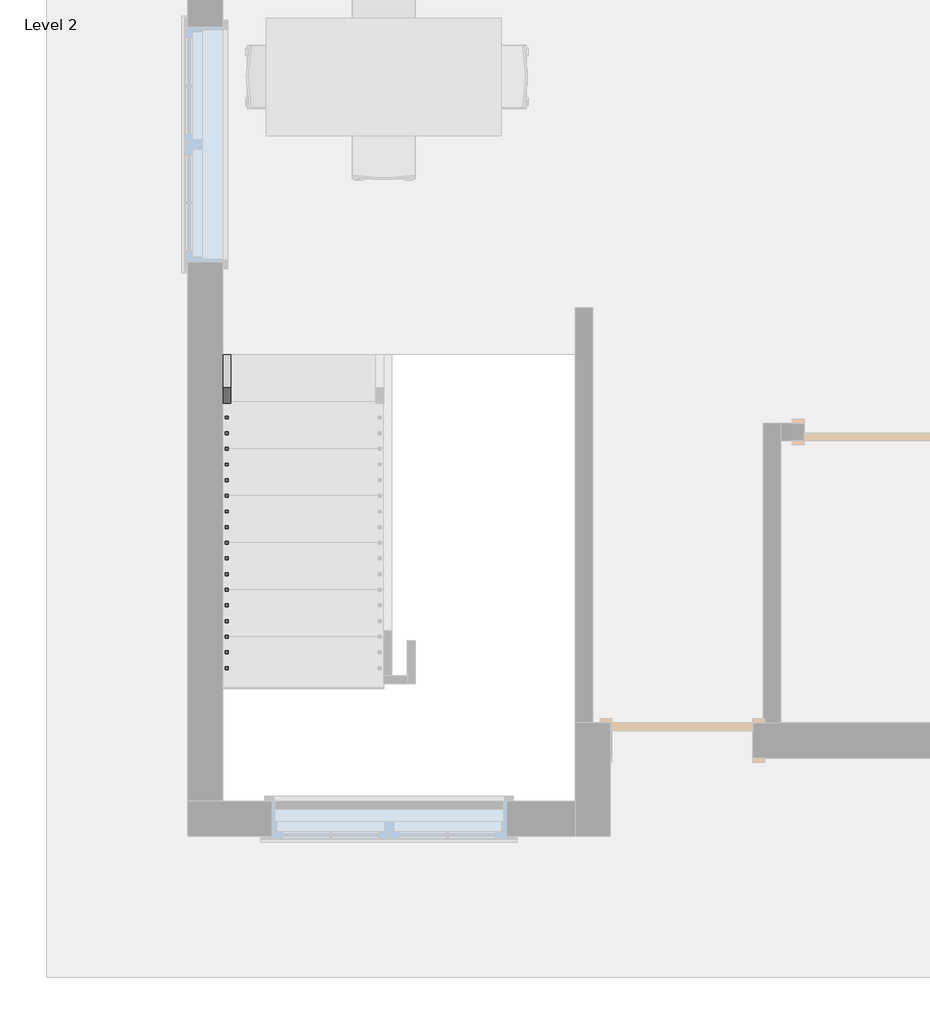
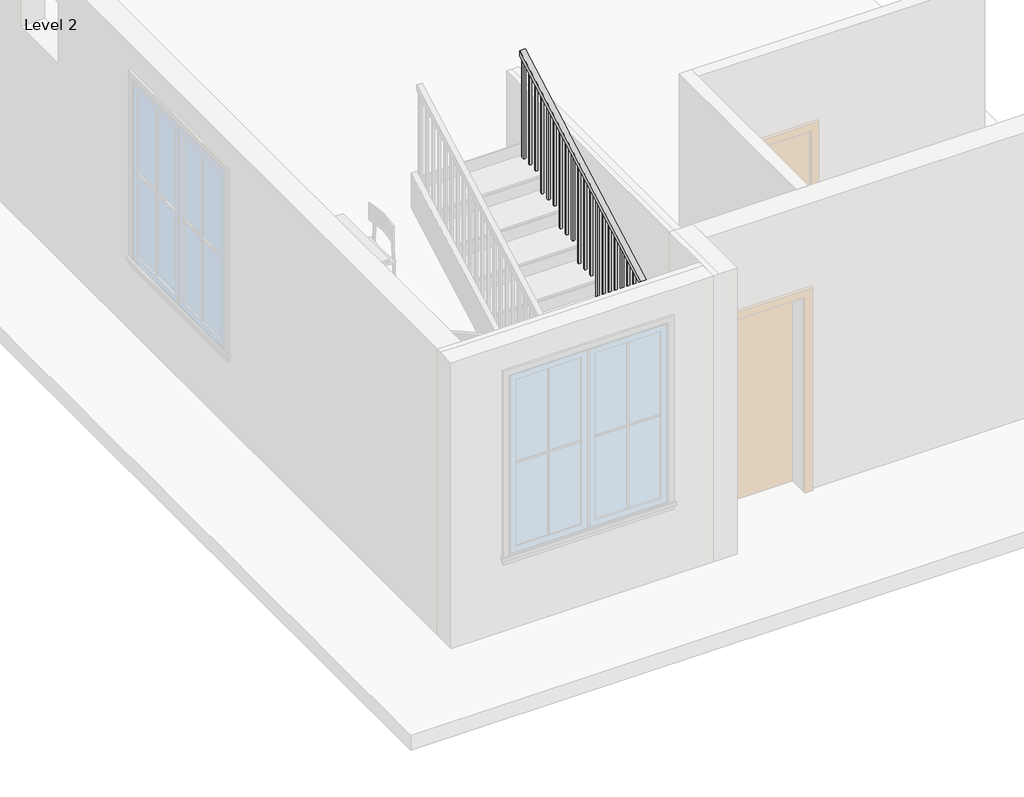
# One storey, part 2 of 3: 1 railing.
"""IFC4 building model written with IfcOpenShell, lengths in millimetres."""

from ifc_helpers import new_model, si_unit, frame, origin, place, context, project, spatial, polyline, outline, extrude, faceted_brep, element, save

model = new_model("IFC4")

# Units and contexts
model_context = context("Model", 3, world=origin())
ifc_project = project(units=[si_unit("LENGTHUNIT", "METRE", prefix="MILLI")], contexts=[model_context])

# Site, building, storey
site = spatial("IfcSite", under=ifc_project)
building = spatial("IfcBuilding", under=site)
storey = spatial("IfcBuildingStorey", under=building, Name="Level 2", Elevation=3048.0)

# Railing
placement = place(None, origin())
element("IfcRailing", 1, ObjectType="Handrail - Rectangular", at=placement, inside=storey, context=model_context, shape_type="SolidModel", body=[
    faceted_brep([(-4181.480864, -3571.6080018, 4131.7333333), (-4181.480864, -3571.6080018, 4073.620221), (-4232.280864, -3571.6080018, 4073.620221), (-4232.280864, -3571.6080018, 4131.7333333), (-4181.480864, -5705.2080018, 5317.0666667), (-4181.480864, -5718.371604, 5266.2666667), (-4232.280864, -5718.371604, 5266.2666667), (-4232.280864, -5705.2080018, 5317.0666667), (-4181.480864, -6416.4080018, 5317.0666667), (-4181.480864, -6416.4080018, 5266.2666667), (-4232.280864, -6467.2080018, 5266.2666667), (-4232.280864, -6467.2080018, 5317.0666667), (-1997.080864, -6416.4080018, 5317.0666667), (-1997.080864, -6416.4080018, 5266.2666667), (-1946.280864, -6467.2080018, 5266.2666667), (-1946.280864, -6467.2080018, 5317.0666667), (-1997.080864, -5705.2080018, 5317.0666667), (-1997.080864, -5692.0443995, 5266.2666667), (-1946.280864, -5692.0443995, 5266.2666667), (-1946.280864, -5705.2080018, 5317.0666667), (-1997.080864, -3571.6080018, 6502.4), (-1946.280864, -3571.6080018, 6502.4), (-1946.280864, -3571.6080018, 6444.2868876), (-1997.080864, -3571.6080018, 6444.2868876)], [[[0, 1, 2, 3]], [[1, 0, 4, 5]], [[2, 1, 5, 6]], [[3, 2, 6, 7]], [[0, 3, 7, 4]], [[5, 4, 8, 9]], [[6, 5, 9, 10]], [[7, 6, 10, 11]], [[4, 7, 11, 8]], [[9, 8, 12, 13]], [[10, 9, 13, 14]], [[11, 10, 14, 15]], [[8, 11, 15, 12]], [[13, 12, 16, 17]], [[14, 13, 17, 18]], [[15, 14, 18, 19]], [[12, 15, 19, 16]], [[20, 21, 22, 23]], [[17, 16, 20, 23]], [[18, 17, 23, 22]], [[19, 18, 22, 21]], [[16, 19, 21, 20]]]),
    extrude(outline(polyline([(-3606.5330018, 6424.8841099), (-3587.4830018, 6435.4674432), (-3587.4830018, 5418.6666667), (-3606.5330018, 5418.6666667), (-3606.5330018, 6424.8841099)])), frame((-1981.205864, 0.0, 0.0), z_axis=(1.0, 0.0, 0.0), x_axis=(0.0, 1.0, 0.0)), (0.0, 0.0, 1.0), 19.05),
    extrude(outline(polyline([(-3708.1330018, 6368.4396654), (-3689.0830018, 6379.0229988), (-3689.0830018, 5418.6666667), (-3708.1330018, 5418.6666667), (-3708.1330018, 6368.4396654)])), frame((-1981.205864, 0.0, 0.0), z_axis=(1.0, 0.0, 0.0), x_axis=(0.0, 1.0, 0.0)), (0.0, 0.0, 1.0), 19.05),
    extrude(outline(polyline([(-3809.7330018, 6311.995221), (-3790.6830018, 6322.5785543), (-3790.6830018, 5418.6666667), (-3809.7330018, 5418.6666667), (-3809.7330018, 6311.995221)])), frame((-1981.205864, 0.0, 0.0), z_axis=(1.0, 0.0, 0.0), x_axis=(0.0, 1.0, 0.0)), (0.0, 0.0, 1.0), 19.05),
    extrude(outline(polyline([(-3911.3330018, 6255.5507765), (-3892.2830018, 6266.1341099), (-3892.2830018, 5249.3333333), (-3911.3330018, 5249.3333333), (-3911.3330018, 6255.5507765)])), frame((-1981.205864, 0.0, 0.0), z_axis=(1.0, 0.0, 0.0), x_axis=(0.0, 1.0, 0.0)), (0.0, 0.0, 1.0), 19.05),
    extrude(outline(polyline([(-4012.9330018, 6199.1063321), (-3993.8830018, 6209.6896654), (-3993.8830018, 5249.3333333), (-4012.9330018, 5249.3333333), (-4012.9330018, 6199.1063321)])), frame((-1981.205864, 0.0, 0.0), z_axis=(1.0, 0.0, 0.0), x_axis=(0.0, 1.0, 0.0)), (0.0, 0.0, 1.0), 19.05),
    extrude(outline(polyline([(-4114.5330018, 6142.6618876), (-4095.4830018, 6153.245221), (-4095.4830018, 5249.3333333), (-4114.5330018, 5249.3333333), (-4114.5330018, 6142.6618876)])), frame((-1981.205864, 0.0, 0.0), z_axis=(1.0, 0.0, 0.0), x_axis=(0.0, 1.0, 0.0)), (0.0, 0.0, 1.0), 19.05),
    extrude(outline(polyline([(-4216.1330018, 6086.2174432), (-4197.0830018, 6096.8007765), (-4197.0830018, 5080.0), (-4216.1330018, 5080.0), (-4216.1330018, 6086.2174432)])), frame((-1981.205864, 0.0, 0.0), z_axis=(1.0, 0.0, 0.0), x_axis=(0.0, 1.0, 0.0)), (0.0, 0.0, 1.0), 19.05),
    extrude(outline(polyline([(-4317.7330018, 6029.7729988), (-4298.6830018, 6040.3563321), (-4298.6830018, 5080.0), (-4317.7330018, 5080.0), (-4317.7330018, 6029.7729988)])), frame((-1981.205864, 0.0, 0.0), z_axis=(1.0, 0.0, 0.0), x_axis=(0.0, 1.0, 0.0)), (0.0, 0.0, 1.0), 19.05),
    extrude(outline(polyline([(-4419.3330018, 5973.3285543), (-4400.2830018, 5983.9118876), (-4400.2830018, 5080.0), (-4419.3330018, 5080.0), (-4419.3330018, 5973.3285543)])), frame((-1981.205864, 0.0, 0.0), z_axis=(1.0, 0.0, 0.0), x_axis=(0.0, 1.0, 0.0)), (0.0, 0.0, 1.0), 19.05),
    extrude(outline(polyline([(-4520.9330018, 5916.8841099), (-4501.8830018, 5927.4674432), (-4501.8830018, 4910.6666667), (-4520.9330018, 4910.6666667), (-4520.9330018, 5916.8841099)])), frame((-1981.205864, 0.0, 0.0), z_axis=(1.0, 0.0, 0.0), x_axis=(0.0, 1.0, 0.0)), (0.0, 0.0, 1.0), 19.05),
    extrude(outline(polyline([(-4622.5330018, 5860.4396654), (-4603.4830018, 5871.0229988), (-4603.4830018, 4910.6666667), (-4622.5330018, 4910.6666667), (-4622.5330018, 5860.4396654)])), frame((-1981.205864, 0.0, 0.0), z_axis=(1.0, 0.0, 0.0), x_axis=(0.0, 1.0, 0.0)), (0.0, 0.0, 1.0), 19.05),
    extrude(outline(polyline([(-4724.1330018, 5803.995221), (-4705.0830018, 5814.5785543), (-4705.0830018, 4910.6666667), (-4724.1330018, 4910.6666667), (-4724.1330018, 5803.995221)])), frame((-1981.205864, 0.0, 0.0), z_axis=(1.0, 0.0, 0.0), x_axis=(0.0, 1.0, 0.0)), (0.0, 0.0, 1.0), 19.05),
    extrude(outline(polyline([(-4825.7330018, 5747.5507765), (-4806.6830018, 5758.1341099), (-4806.6830018, 4741.3333333), (-4825.7330018, 4741.3333333), (-4825.7330018, 5747.5507765)])), frame((-1981.205864, 0.0, 0.0), z_axis=(1.0, 0.0, 0.0), x_axis=(0.0, 1.0, 0.0)), (0.0, 0.0, 1.0), 19.05),
    extrude(outline(polyline([(-4927.3330018, 5691.1063321), (-4908.2830018, 5701.6896654), (-4908.2830018, 4741.3333333), (-4927.3330018, 4741.3333333), (-4927.3330018, 5691.1063321)])), frame((-1981.205864, 0.0, 0.0), z_axis=(1.0, 0.0, 0.0), x_axis=(0.0, 1.0, 0.0)), (0.0, 0.0, 1.0), 19.05),
    extrude(outline(polyline([(-5028.9330018, 5634.6618876), (-5009.8830018, 5645.245221), (-5009.8830018, 4741.3333333), (-5028.9330018, 4741.3333333), (-5028.9330018, 5634.6618876)])), frame((-1981.205864, 0.0, 0.0), z_axis=(1.0, 0.0, 0.0), x_axis=(0.0, 1.0, 0.0)), (0.0, 0.0, 1.0), 19.05),
    extrude(outline(polyline([(-5130.5330018, 5578.2174432), (-5111.4830018, 5588.8007765), (-5111.4830018, 4572.0), (-5130.5330018, 4572.0), (-5130.5330018, 5578.2174432)])), frame((-1981.205864, 0.0, 0.0), z_axis=(1.0, 0.0, 0.0), x_axis=(0.0, 1.0, 0.0)), (0.0, 0.0, 1.0), 19.05),
    extrude(outline(polyline([(-5232.1330018, 5521.7729988), (-5213.0830018, 5532.3563321), (-5213.0830018, 4572.0), (-5232.1330018, 4572.0), (-5232.1330018, 5521.7729988)])), frame((-1981.205864, 0.0, 0.0), z_axis=(1.0, 0.0, 0.0), x_axis=(0.0, 1.0, 0.0)), (0.0, 0.0, 1.0), 19.05),
    extrude(outline(polyline([(-5333.7330018, 5465.3285543), (-5314.6830018, 5475.9118876), (-5314.6830018, 4572.0), (-5333.7330018, 4572.0), (-5333.7330018, 5465.3285543)])), frame((-1981.205864, 0.0, 0.0), z_axis=(1.0, 0.0, 0.0), x_axis=(0.0, 1.0, 0.0)), (0.0, 0.0, 1.0), 19.05),
    extrude(outline(polyline([(-5435.3330018, 5408.8841099), (-5416.2830018, 5419.4674432), (-5416.2830018, 4402.6666667), (-5435.3330018, 4402.6666667), (-5435.3330018, 5408.8841099)])), frame((-1981.205864, 0.0, 0.0), z_axis=(1.0, 0.0, 0.0), x_axis=(0.0, 1.0, 0.0)), (0.0, 0.0, 1.0), 19.05),
    extrude(outline(polyline([(-5536.9330018, 5352.4396654), (-5517.8830018, 5363.0229988), (-5517.8830018, 4402.6666667), (-5536.9330018, 4402.6666667), (-5536.9330018, 5352.4396654)])), frame((-1981.205864, 0.0, 0.0), z_axis=(1.0, 0.0, 0.0), x_axis=(0.0, 1.0, 0.0)), (0.0, 0.0, 1.0), 19.05),
    extrude(outline(polyline([(-5638.5330018, 5295.995221), (-5619.4830018, 5306.5785543), (-5619.4830018, 4402.6666667), (-5638.5330018, 4402.6666667), (-5638.5330018, 5295.995221)])), frame((-1981.205864, 0.0, 0.0), z_axis=(1.0, 0.0, 0.0), x_axis=(0.0, 1.0, 0.0)), (0.0, 0.0, 1.0), 19.05),
    extrude(outline(polyline([(-1962.155864, -5740.1330018), (-1981.205864, -5740.1330018), (-1981.205864, -5721.0830018), (-1962.155864, -5721.0830018), (-1962.155864, -5740.1330018)])), frame((0.0, 0.0, 4402.6666667), z_axis=(0.0, 0.0, 1.0), x_axis=(1.0, 0.0, 0.0)), (0.0, 0.0, 1.0), 863.6),
    extrude(outline(polyline([(-1962.155864, -5841.7330018), (-1981.205864, -5841.7330018), (-1981.205864, -5822.6830018), (-1962.155864, -5822.6830018), (-1962.155864, -5841.7330018)])), frame((0.0, 0.0, 4402.6666667), z_axis=(0.0, 0.0, 1.0), x_axis=(1.0, 0.0, 0.0)), (0.0, 0.0, 1.0), 863.6),
    extrude(outline(polyline([(-1962.155864, -5943.3330018), (-1981.205864, -5943.3330018), (-1981.205864, -5924.2830018), (-1962.155864, -5924.2830018), (-1962.155864, -5943.3330018)])), frame((0.0, 0.0, 4402.6666667), z_axis=(0.0, 0.0, 1.0), x_axis=(1.0, 0.0, 0.0)), (0.0, 0.0, 1.0), 863.6),
    extrude(outline(polyline([(-1962.155864, -6044.9330018), (-1981.205864, -6044.9330018), (-1981.205864, -6025.8830018), (-1962.155864, -6025.8830018), (-1962.155864, -6044.9330018)])), frame((0.0, 0.0, 4402.6666667), z_axis=(0.0, 0.0, 1.0), x_axis=(1.0, 0.0, 0.0)), (0.0, 0.0, 1.0), 863.6),
    extrude(outline(polyline([(-1962.155864, -6146.5330018), (-1981.205864, -6146.5330018), (-1981.205864, -6127.4830018), (-1962.155864, -6127.4830018), (-1962.155864, -6146.5330018)])), frame((0.0, 0.0, 4402.6666667), z_axis=(0.0, 0.0, 1.0), x_axis=(1.0, 0.0, 0.0)), (0.0, 0.0, 1.0), 863.6),
    extrude(outline(polyline([(-1962.155864, -6248.1330018), (-1981.205864, -6248.1330018), (-1981.205864, -6229.0830018), (-1962.155864, -6229.0830018), (-1962.155864, -6248.1330018)])), frame((0.0, 0.0, 4402.6666667), z_axis=(0.0, 0.0, 1.0), x_axis=(1.0, 0.0, 0.0)), (0.0, 0.0, 1.0), 863.6),
    extrude(outline(polyline([(-1962.155864, -6349.7330018), (-1981.205864, -6349.7330018), (-1981.205864, -6330.6830018), (-1962.155864, -6330.6830018), (-1962.155864, -6349.7330018)])), frame((0.0, 0.0, 4402.6666667), z_axis=(0.0, 0.0, 1.0), x_axis=(1.0, 0.0, 0.0)), (0.0, 0.0, 1.0), 863.6),
    extrude(outline(polyline([(-2082.805864, -6451.3330018), (-2082.805864, -6432.2830018), (-2063.755864, -6432.2830018), (-2063.755864, -6451.3330018), (-2082.805864, -6451.3330018)])), frame((0.0, 0.0, 4402.6666667), z_axis=(0.0, 0.0, 1.0), x_axis=(1.0, 0.0, 0.0)), (0.0, 0.0, 1.0), 863.6),
    extrude(outline(polyline([(-2184.405864, -6451.3330018), (-2184.405864, -6432.2830018), (-2165.355864, -6432.2830018), (-2165.355864, -6451.3330018), (-2184.405864, -6451.3330018)])), frame((0.0, 0.0, 4402.6666667), z_axis=(0.0, 0.0, 1.0), x_axis=(1.0, 0.0, 0.0)), (0.0, 0.0, 1.0), 863.6),
    extrude(outline(polyline([(-2286.005864, -6451.3330018), (-2286.005864, -6432.2830018), (-2266.955864, -6432.2830018), (-2266.955864, -6451.3330018), (-2286.005864, -6451.3330018)])), frame((0.0, 0.0, 4402.6666667), z_axis=(0.0, 0.0, 1.0), x_axis=(1.0, 0.0, 0.0)), (0.0, 0.0, 1.0), 863.6),
    extrude(outline(polyline([(-2387.605864, -6451.3330018), (-2387.605864, -6432.2830018), (-2368.555864, -6432.2830018), (-2368.555864, -6451.3330018), (-2387.605864, -6451.3330018)])), frame((0.0, 0.0, 4402.6666667), z_axis=(0.0, 0.0, 1.0), x_axis=(1.0, 0.0, 0.0)), (0.0, 0.0, 1.0), 863.6),
    extrude(outline(polyline([(-2489.205864, -6451.3330018), (-2489.205864, -6432.2830018), (-2470.155864, -6432.2830018), (-2470.155864, -6451.3330018), (-2489.205864, -6451.3330018)])), frame((0.0, 0.0, 4402.6666667), z_axis=(0.0, 0.0, 1.0), x_axis=(1.0, 0.0, 0.0)), (0.0, 0.0, 1.0), 863.6),
    extrude(outline(polyline([(-2590.805864, -6451.3330018), (-2590.805864, -6432.2830018), (-2571.755864, -6432.2830018), (-2571.755864, -6451.3330018), (-2590.805864, -6451.3330018)])), frame((0.0, 0.0, 4402.6666667), z_axis=(0.0, 0.0, 1.0), x_axis=(1.0, 0.0, 0.0)), (0.0, 0.0, 1.0), 863.6),
    extrude(outline(polyline([(-2692.405864, -6451.3330018), (-2692.405864, -6432.2830018), (-2673.355864, -6432.2830018), (-2673.355864, -6451.3330018), (-2692.405864, -6451.3330018)])), frame((0.0, 0.0, 4402.6666667), z_axis=(0.0, 0.0, 1.0), x_axis=(1.0, 0.0, 0.0)), (0.0, 0.0, 1.0), 863.6),
    extrude(outline(polyline([(-2794.005864, -6451.3330018), (-2794.005864, -6432.2830018), (-2774.955864, -6432.2830018), (-2774.955864, -6451.3330018), (-2794.005864, -6451.3330018)])), frame((0.0, 0.0, 4402.6666667), z_axis=(0.0, 0.0, 1.0), x_axis=(1.0, 0.0, 0.0)), (0.0, 0.0, 1.0), 863.6),
    extrude(outline(polyline([(-2895.605864, -6451.3330018), (-2895.605864, -6432.2830018), (-2876.555864, -6432.2830018), (-2876.555864, -6451.3330018), (-2895.605864, -6451.3330018)])), frame((0.0, 0.0, 4402.6666667), z_axis=(0.0, 0.0, 1.0), x_axis=(1.0, 0.0, 0.0)), (0.0, 0.0, 1.0), 863.6),
    extrude(outline(polyline([(-2997.205864, -6451.3330018), (-2997.205864, -6432.2830018), (-2978.155864, -6432.2830018), (-2978.155864, -6451.3330018), (-2997.205864, -6451.3330018)])), frame((0.0, 0.0, 4402.6666667), z_axis=(0.0, 0.0, 1.0), x_axis=(1.0, 0.0, 0.0)), (0.0, 0.0, 1.0), 863.6),
    extrude(outline(polyline([(-3098.805864, -6451.3330018), (-3098.805864, -6432.2830018), (-3079.755864, -6432.2830018), (-3079.755864, -6451.3330018), (-3098.805864, -6451.3330018)])), frame((0.0, 0.0, 4402.6666667), z_axis=(0.0, 0.0, 1.0), x_axis=(1.0, 0.0, 0.0)), (0.0, 0.0, 1.0), 863.6),
    extrude(outline(polyline([(-3200.405864, -6451.3330018), (-3200.405864, -6432.2830018), (-3181.355864, -6432.2830018), (-3181.355864, -6451.3330018), (-3200.405864, -6451.3330018)])), frame((0.0, 0.0, 4402.6666667), z_axis=(0.0, 0.0, 1.0), x_axis=(1.0, 0.0, 0.0)), (0.0, 0.0, 1.0), 863.6),
    extrude(outline(polyline([(-3302.005864, -6451.3330018), (-3302.005864, -6432.2830018), (-3282.955864, -6432.2830018), (-3282.955864, -6451.3330018), (-3302.005864, -6451.3330018)])), frame((0.0, 0.0, 4402.6666667), z_axis=(0.0, 0.0, 1.0), x_axis=(1.0, 0.0, 0.0)), (0.0, 0.0, 1.0), 863.6),
    extrude(outline(polyline([(-3403.605864, -6451.3330018), (-3403.605864, -6432.2830018), (-3384.555864, -6432.2830018), (-3384.555864, -6451.3330018), (-3403.605864, -6451.3330018)])), frame((0.0, 0.0, 4402.6666667), z_axis=(0.0, 0.0, 1.0), x_axis=(1.0, 0.0, 0.0)), (0.0, 0.0, 1.0), 863.6),
    extrude(outline(polyline([(-3505.205864, -6451.3330018), (-3505.205864, -6432.2830018), (-3486.155864, -6432.2830018), (-3486.155864, -6451.3330018), (-3505.205864, -6451.3330018)])), frame((0.0, 0.0, 4402.6666667), z_axis=(0.0, 0.0, 1.0), x_axis=(1.0, 0.0, 0.0)), (0.0, 0.0, 1.0), 863.6),
    extrude(outline(polyline([(-3606.805864, -6451.3330018), (-3606.805864, -6432.2830018), (-3587.755864, -6432.2830018), (-3587.755864, -6451.3330018), (-3606.805864, -6451.3330018)])), frame((0.0, 0.0, 4402.6666667), z_axis=(0.0, 0.0, 1.0), x_axis=(1.0, 0.0, 0.0)), (0.0, 0.0, 1.0), 863.6),
    extrude(outline(polyline([(-3708.405864, -6451.3330018), (-3708.405864, -6432.2830018), (-3689.355864, -6432.2830018), (-3689.355864, -6451.3330018), (-3708.405864, -6451.3330018)])), frame((0.0, 0.0, 4402.6666667), z_axis=(0.0, 0.0, 1.0), x_axis=(1.0, 0.0, 0.0)), (0.0, 0.0, 1.0), 863.6),
    extrude(outline(polyline([(-3810.005864, -6451.3330018), (-3810.005864, -6432.2830018), (-3790.955864, -6432.2830018), (-3790.955864, -6451.3330018), (-3810.005864, -6451.3330018)])), frame((0.0, 0.0, 4402.6666667), z_axis=(0.0, 0.0, 1.0), x_axis=(1.0, 0.0, 0.0)), (0.0, 0.0, 1.0), 863.6),
    extrude(outline(polyline([(-3911.605864, -6451.3330018), (-3911.605864, -6432.2830018), (-3892.555864, -6432.2830018), (-3892.555864, -6451.3330018), (-3911.605864, -6451.3330018)])), frame((0.0, 0.0, 4402.6666667), z_axis=(0.0, 0.0, 1.0), x_axis=(1.0, 0.0, 0.0)), (0.0, 0.0, 1.0), 863.6),
    extrude(outline(polyline([(-4013.205864, -6451.3330018), (-4013.205864, -6432.2830018), (-3994.155864, -6432.2830018), (-3994.155864, -6451.3330018), (-4013.205864, -6451.3330018)])), frame((0.0, 0.0, 4402.6666667), z_axis=(0.0, 0.0, 1.0), x_axis=(1.0, 0.0, 0.0)), (0.0, 0.0, 1.0), 863.6),
    extrude(outline(polyline([(-4114.805864, -6451.3330018), (-4114.805864, -6432.2830018), (-4095.755864, -6432.2830018), (-4095.755864, -6451.3330018), (-4114.805864, -6451.3330018)])), frame((0.0, 0.0, 4402.6666667), z_axis=(0.0, 0.0, 1.0), x_axis=(1.0, 0.0, 0.0)), (0.0, 0.0, 1.0), 863.6),
    extrude(outline(polyline([(-4216.405864, -6406.8830018), (-4197.355864, -6406.8830018), (-4197.355864, -6425.9330018), (-4216.405864, -6425.9330018), (-4216.405864, -6406.8830018)])), frame((0.0, 0.0, 4402.6666667), z_axis=(0.0, 0.0, 1.0), x_axis=(1.0, 0.0, 0.0)), (0.0, 0.0, 1.0), 863.6),
    extrude(outline(polyline([(-4216.405864, -6305.2830018), (-4197.355864, -6305.2830018), (-4197.355864, -6324.3330018), (-4216.405864, -6324.3330018), (-4216.405864, -6305.2830018)])), frame((0.0, 0.0, 4402.6666667), z_axis=(0.0, 0.0, 1.0), x_axis=(1.0, 0.0, 0.0)), (0.0, 0.0, 1.0), 863.6),
    extrude(outline(polyline([(-4216.405864, -6203.6830018), (-4197.355864, -6203.6830018), (-4197.355864, -6222.7330018), (-4216.405864, -6222.7330018), (-4216.405864, -6203.6830018)])), frame((0.0, 0.0, 4402.6666667), z_axis=(0.0, 0.0, 1.0), x_axis=(1.0, 0.0, 0.0)), (0.0, 0.0, 1.0), 863.6),
    extrude(outline(polyline([(-4216.405864, -6102.0830018), (-4197.355864, -6102.0830018), (-4197.355864, -6121.1330018), (-4216.405864, -6121.1330018), (-4216.405864, -6102.0830018)])), frame((0.0, 0.0, 4402.6666667), z_axis=(0.0, 0.0, 1.0), x_axis=(1.0, 0.0, 0.0)), (0.0, 0.0, 1.0), 863.6),
    extrude(outline(polyline([(-4216.405864, -6000.4830018), (-4197.355864, -6000.4830018), (-4197.355864, -6019.5330018), (-4216.405864, -6019.5330018), (-4216.405864, -6000.4830018)])), frame((0.0, 0.0, 4402.6666667), z_axis=(0.0, 0.0, 1.0), x_axis=(1.0, 0.0, 0.0)), (0.0, 0.0, 1.0), 863.6),
    extrude(outline(polyline([(-4216.405864, -5898.8830018), (-4197.355864, -5898.8830018), (-4197.355864, -5917.9330018), (-4216.405864, -5917.9330018), (-4216.405864, -5898.8830018)])), frame((0.0, 0.0, 4402.6666667), z_axis=(0.0, 0.0, 1.0), x_axis=(1.0, 0.0, 0.0)), (0.0, 0.0, 1.0), 863.6),
    extrude(outline(polyline([(-4216.405864, -5797.2830018), (-4197.355864, -5797.2830018), (-4197.355864, -5816.3330018), (-4216.405864, -5816.3330018), (-4216.405864, -5797.2830018)])), frame((0.0, 0.0, 4402.6666667), z_axis=(0.0, 0.0, 1.0), x_axis=(1.0, 0.0, 0.0)), (0.0, 0.0, 1.0), 863.6),
    extrude(outline(polyline([(-5714.7330018, 5264.245221), (-5695.6830018, 5253.6618876), (-5695.6830018, 4402.6666667), (-5714.7330018, 4402.6666667), (-5714.7330018, 5264.245221)])), frame((-4216.405864, 0.0, 0.0), z_axis=(1.0, 0.0, 0.0), x_axis=(0.0, 1.0, 0.0)), (0.0, 0.0, 1.0), 19.05),
    extrude(outline(polyline([(-5613.1330018, 5207.8007765), (-5594.0830018, 5197.2174432), (-5594.0830018, 4233.3333333), (-5613.1330018, 4233.3333333), (-5613.1330018, 5207.8007765)])), frame((-4216.405864, 0.0, 0.0), z_axis=(1.0, 0.0, 0.0), x_axis=(0.0, 1.0, 0.0)), (0.0, 0.0, 1.0), 19.05),
    extrude(outline(polyline([(-5511.5330018, 5151.3563321), (-5492.4830018, 5140.7729988), (-5492.4830018, 4233.3333333), (-5511.5330018, 4233.3333333), (-5511.5330018, 5151.3563321)])), frame((-4216.405864, 0.0, 0.0), z_axis=(1.0, 0.0, 0.0), x_axis=(0.0, 1.0, 0.0)), (0.0, 0.0, 1.0), 19.05),
    extrude(outline(polyline([(-5409.9330018, 5094.9118876), (-5390.8830018, 5084.3285543), (-5390.8830018, 4233.3333333), (-5409.9330018, 4233.3333333), (-5409.9330018, 5094.9118876)])), frame((-4216.405864, 0.0, 0.0), z_axis=(1.0, 0.0, 0.0), x_axis=(0.0, 1.0, 0.0)), (0.0, 0.0, 1.0), 19.05),
    extrude(outline(polyline([(-5308.3330018, 5038.4674432), (-5289.2830018, 5027.8841099), (-5289.2830018, 4064.0), (-5308.3330018, 4064.0), (-5308.3330018, 5038.4674432)])), frame((-4216.405864, 0.0, 0.0), z_axis=(1.0, 0.0, 0.0), x_axis=(0.0, 1.0, 0.0)), (0.0, 0.0, 1.0), 19.05),
    extrude(outline(polyline([(-5206.7330018, 4982.0229988), (-5187.6830018, 4971.4396654), (-5187.6830018, 4064.0), (-5206.7330018, 4064.0), (-5206.7330018, 4982.0229988)])), frame((-4216.405864, 0.0, 0.0), z_axis=(1.0, 0.0, 0.0), x_axis=(0.0, 1.0, 0.0)), (0.0, 0.0, 1.0), 19.05),
    extrude(outline(polyline([(-5105.1330018, 4925.5785543), (-5086.0830018, 4914.995221), (-5086.0830018, 4064.0), (-5105.1330018, 4064.0), (-5105.1330018, 4925.5785543)])), frame((-4216.405864, 0.0, 0.0), z_axis=(1.0, 0.0, 0.0), x_axis=(0.0, 1.0, 0.0)), (0.0, 0.0, 1.0), 19.05),
    extrude(outline(polyline([(-5003.5330018, 4869.1341099), (-4984.4830018, 4858.5507765), (-4984.4830018, 3894.6666667), (-5003.5330018, 3894.6666667), (-5003.5330018, 4869.1341099)])), frame((-4216.405864, 0.0, 0.0), z_axis=(1.0, 0.0, 0.0), x_axis=(0.0, 1.0, 0.0)), (0.0, 0.0, 1.0), 19.05),
    extrude(outline(polyline([(-4901.9330018, 4812.6896654), (-4882.8830018, 4802.1063321), (-4882.8830018, 3894.6666667), (-4901.9330018, 3894.6666667), (-4901.9330018, 4812.6896654)])), frame((-4216.405864, 0.0, 0.0), z_axis=(1.0, 0.0, 0.0), x_axis=(0.0, 1.0, 0.0)), (0.0, 0.0, 1.0), 19.05),
    extrude(outline(polyline([(-4800.3330018, 4756.245221), (-4781.2830018, 4745.6618876), (-4781.2830018, 3894.6666667), (-4800.3330018, 3894.6666667), (-4800.3330018, 4756.245221)])), frame((-4216.405864, 0.0, 0.0), z_axis=(1.0, 0.0, 0.0), x_axis=(0.0, 1.0, 0.0)), (0.0, 0.0, 1.0), 19.05),
    extrude(outline(polyline([(-4698.7330018, 4699.8007765), (-4679.6830018, 4689.2174432), (-4679.6830018, 3725.3333333), (-4698.7330018, 3725.3333333), (-4698.7330018, 4699.8007765)])), frame((-4216.405864, 0.0, 0.0), z_axis=(1.0, 0.0, 0.0), x_axis=(0.0, 1.0, 0.0)), (0.0, 0.0, 1.0), 19.05),
    extrude(outline(polyline([(-4597.1330018, 4643.3563321), (-4578.0830018, 4632.7729988), (-4578.0830018, 3725.3333333), (-4597.1330018, 3725.3333333), (-4597.1330018, 4643.3563321)])), frame((-4216.405864, 0.0, 0.0), z_axis=(1.0, 0.0, 0.0), x_axis=(0.0, 1.0, 0.0)), (0.0, 0.0, 1.0), 19.05),
    extrude(outline(polyline([(-4495.5330018, 4586.9118876), (-4476.4830018, 4576.3285543), (-4476.4830018, 3725.3333333), (-4495.5330018, 3725.3333333), (-4495.5330018, 4586.9118876)])), frame((-4216.405864, 0.0, 0.0), z_axis=(1.0, 0.0, 0.0), x_axis=(0.0, 1.0, 0.0)), (0.0, 0.0, 1.0), 19.05),
    extrude(outline(polyline([(-4393.9330018, 4530.4674432), (-4374.8830018, 4519.8841099), (-4374.8830018, 3556.0), (-4393.9330018, 3556.0), (-4393.9330018, 4530.4674432)])), frame((-4216.405864, 0.0, 0.0), z_axis=(1.0, 0.0, 0.0), x_axis=(0.0, 1.0, 0.0)), (0.0, 0.0, 1.0), 19.05),
    extrude(outline(polyline([(-4292.3330018, 4474.0229988), (-4273.2830018, 4463.4396654), (-4273.2830018, 3556.0), (-4292.3330018, 3556.0), (-4292.3330018, 4474.0229988)])), frame((-4216.405864, 0.0, 0.0), z_axis=(1.0, 0.0, 0.0), x_axis=(0.0, 1.0, 0.0)), (0.0, 0.0, 1.0), 19.05),
    extrude(outline(polyline([(-4190.7330018, 4417.5785543), (-4171.6830018, 4406.995221), (-4171.6830018, 3556.0), (-4190.7330018, 3556.0), (-4190.7330018, 4417.5785543)])), frame((-4216.405864, 0.0, 0.0), z_axis=(1.0, 0.0, 0.0), x_axis=(0.0, 1.0, 0.0)), (0.0, 0.0, 1.0), 19.05),
    extrude(outline(polyline([(-4089.1330018, 4361.1341099), (-4070.0830018, 4350.5507765), (-4070.0830018, 3386.6666667), (-4089.1330018, 3386.6666667), (-4089.1330018, 4361.1341099)])), frame((-4216.405864, 0.0, 0.0), z_axis=(1.0, 0.0, 0.0), x_axis=(0.0, 1.0, 0.0)), (0.0, 0.0, 1.0), 19.05),
    extrude(outline(polyline([(-3987.5330018, 4304.6896654), (-3968.4830018, 4294.1063321), (-3968.4830018, 3386.6666667), (-3987.5330018, 3386.6666667), (-3987.5330018, 4304.6896654)])), frame((-4216.405864, 0.0, 0.0), z_axis=(1.0, 0.0, 0.0), x_axis=(0.0, 1.0, 0.0)), (0.0, 0.0, 1.0), 19.05),
    extrude(outline(polyline([(-3885.9330018, 4248.245221), (-3866.8830018, 4237.6618876), (-3866.8830018, 3386.6666667), (-3885.9330018, 3386.6666667), (-3885.9330018, 4248.245221)])), frame((-4216.405864, 0.0, 0.0), z_axis=(1.0, 0.0, 0.0), x_axis=(0.0, 1.0, 0.0)), (0.0, 0.0, 1.0), 19.05),
    extrude(outline(polyline([(-3784.3330018, 4191.8007765), (-3765.2830018, 4181.2174432), (-3765.2830018, 3217.3333333), (-3784.3330018, 3217.3333333), (-3784.3330018, 4191.8007765)])), frame((-4216.405864, 0.0, 0.0), z_axis=(1.0, 0.0, 0.0), x_axis=(0.0, 1.0, 0.0)), (0.0, 0.0, 1.0), 19.05),
    extrude(outline(polyline([(-3682.7330018, 4135.3563321), (-3663.6830018, 4124.7729988), (-3663.6830018, 3217.3333333), (-3682.7330018, 3217.3333333), (-3682.7330018, 4135.3563321)])), frame((-4216.405864, 0.0, 0.0), z_axis=(1.0, 0.0, 0.0), x_axis=(0.0, 1.0, 0.0)), (0.0, 0.0, 1.0), 19.05),
    extrude(outline(polyline([(-1981.205864, -6451.3330018), (-1981.205864, -6432.2830018), (-1962.155864, -6432.2830018), (-1962.155864, -6451.3330018), (-1981.205864, -6451.3330018)])), frame((0.0, 0.0, 4402.6666667), z_axis=(0.0, 0.0, 1.0), x_axis=(1.0, 0.0, 0.0)), (0.0, 0.0, 1.0), 863.6),
    extrude(outline(polyline([(-4216.405864, -6432.2830018), (-4197.355864, -6432.2830018), (-4197.355864, -6451.3330018), (-4216.405864, -6451.3330018), (-4216.405864, -6432.2830018)])), frame((0.0, 0.0, 4402.6666667), z_axis=(0.0, 0.0, 1.0), x_axis=(1.0, 0.0, 0.0)), (0.0, 0.0, 1.0), 863.6),
    extrude(outline(polyline([(-3590.6580018, 6433.7035543), (-3571.6080018, 6444.2868876), (-3571.6080018, 5418.6666667), (-3590.6580018, 5418.6666667), (-3590.6580018, 6433.7035543)])), frame((-1981.205864, 0.0, 0.0), z_axis=(1.0, 0.0, 0.0), x_axis=(0.0, 1.0, 0.0)), (0.0, 0.0, 1.0), 19.05),
    extrude(outline(polyline([(-3590.6580018, 4084.2035543), (-3571.6080018, 4073.620221), (-3571.6080018, 3217.3333333), (-3590.6580018, 3217.3333333), (-3590.6580018, 4084.2035543)])), frame((-4216.405864, 0.0, 0.0), z_axis=(1.0, 0.0, 0.0), x_axis=(0.0, 1.0, 0.0)), (0.0, 0.0, 1.0), 19.05),
])

save(model, "model.ifc")

# Revit data of these elements
# Type "Handrail - Rectangular"
#   Assembly Code = "C2010400"
#   built-in parameter 1008612 = 0.0416667 (stored number, unit not read)
#   built-in parameter 1008611 = 0.0416667 (stored number, unit not read)
#   built-in parameter 1008609 = 0.333333 (stored number, unit not read)
#   built-in parameter 1008604 = 0.166667 (stored number, unit not read)
#   built-in parameter 1008603 = 0.166667 (stored number, unit not read)
#   Railing Height = 3' - 0"
#   built-in parameter 1008630 = 2
#   built-in parameter 1008610 = 2
#   built-in parameter 1008618 = Baluster - Square : 3/4"
# Element 1 (IfcRailing, "Handrail - Rectangular")
#   Phase Created = New Construction
